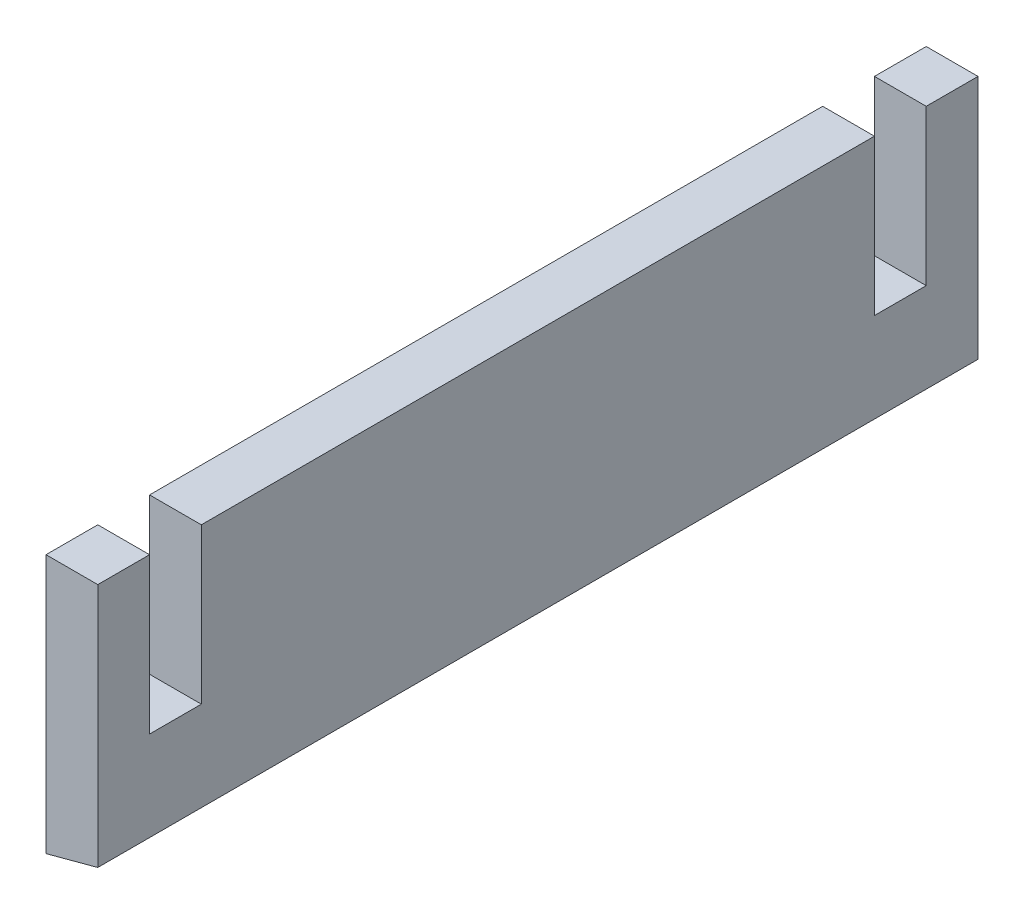
from build123d import *

# Parameters (mm, degrees)
STEP_PLATE_10MM_DEPTH = 5
DRAFT_15DEG_ANGLE     = -15


with BuildPart() as part:
    # Step Plate Profile → Step Plate 10mm (new, symmetric)
    with BuildSketch(Plane(origin=(0, 0, 0), x_dir=(0, 0, -1), z_dir=(1, 0, 0))):
        Polygon((0, 0), (170, 0), (170, 50), (160, 50), (160, 20), (150, 20), (150, 50), (20, 50), (20, 20), (10, 20), (10, 50), (0, 50), align=None)
    extrude(amount=STEP_PLATE_10MM_DEPTH, both=True)

    # Draft 15deg
    draft_15deg_faces = [part.faces().sort_by_distance(p)[0] for p in [
        (0, 0, -85),
    ]]
    draft(draft_15deg_faces, Plane(origin=(-5, 0, 0), x_dir=(0, 0, -1), z_dir=(-1, 0, 0)), DRAFT_15DEG_ANGLE)


solid = part.part
